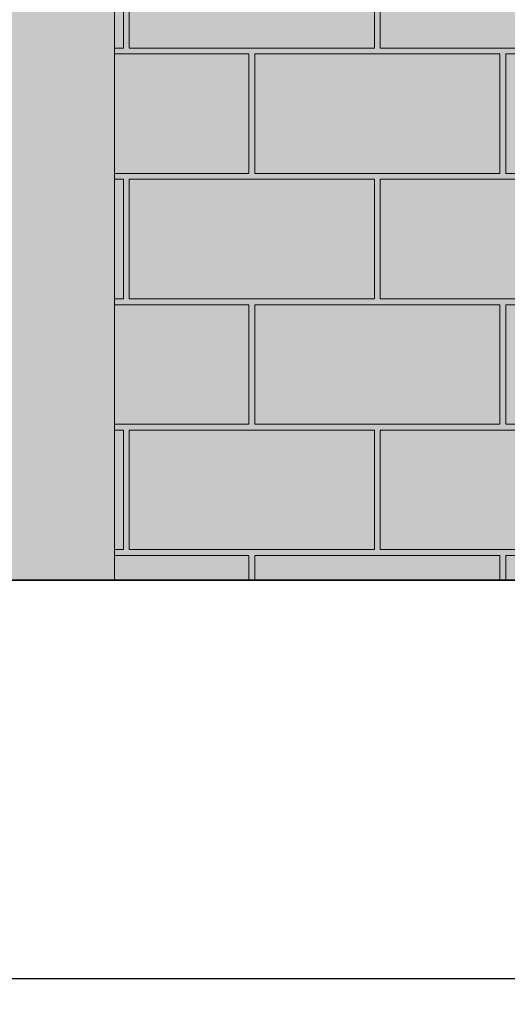
# Model space of a CAD drawing. Units: inches. Extents: x 1704 to 6393, y -157 to 1172.
# Tile 7 of 122: x 1961 to 2035, y -69 to 82. Entities that reach past the tile are written whole.
import ezdxf

# ---------------------------------------------------------------- set-up
doc = ezdxf.new("R2010")
doc.units = ezdxf.units.IN
doc.header["$MEASUREMENT"] = 0
for name, color, linetype, lineweight in [('A-ANNO-DIMS', 7, 'Continuous', 13), ('C-PROP', 7, 'Continuous', 35), ('L-HRDS', 8, 'Continuous', 18), ('L-PVMT-PATT', 8, 'Continuous', 13)]:
    doc.layers.add(name, color=color, linetype=linetype, lineweight=lineweight)
doc.layers.add('L-HRDS-PATT', color=9, linetype='Continuous', lineweight=13, true_color=0xc5c1ba)
doc.layers.add('L-PLNT-PATT', color=253, linetype='Continuous', lineweight=13, true_color=0x9abc8f)
doc.styles.get("Standard").update_dxf_attribs({"font": 'arial.ttf'})
doc.dimstyles.get("Standard").update_dxf_attribs({"dimtxt": 6, "dimasz": 2, "dimexe": 0.18, "dimexo": 0.0625, "dimgap": 0.09, "dimtad": 0, "dimtih": 1, "dimtoh": 1, "dimdec": 1, "dimzin": 0, "dimdsep": 46, "dimlunit": 3, "dimtxsty": 'Standard', "dimblk": 'ARCHTICK', "dimcen": 0.09, "dimadec": 0, "dimazin": 0, "dimtfac": 1, "dimtdec": 1, "dimtofl": 0, "dimtmove": 0, "dimatfit": 3, "dimfxl": 1, "dimtolj": 1, "dimtzin": 0, "dimarcsym": 0})

# ---------------------------------------------------------------- blocks, each defined once
blk = doc.blocks.new('_ArchTick')
at = {"color": 0, "linetype": 'ByBlock', "const_width": 0.15}
blk.add_lwpolyline([(-0.5, -0.5), (0.5, 0.5)], dxfattribs=at)
blk = doc.blocks.new('*D90')
at = {"layer": 'A-ANNO-DIMS', "color": 0, "lineweight": -2, "transparency": 16777216}
for p, q in [((1898.35, -3.85), (1898.35, -64.97)), ((2723.35, -3.85), (2723.35, -64.97)), ((1898.35, -64.79), (2304.1, -64.79)), ((2723.35, -64.79), (2317.59, -64.79))]:
    blk.add_line(p, q, dxfattribs=at)
at = {"layer": 'Defpoints', "color": 0, "lineweight": -3, "transparency": 16777216}
for p in [(1898.35, -3.79), (2723.35, -3.79), (2723.35, -64.79)]:
    blk.add_point(p, dxfattribs=at)
at = {"layer": 'A-ANNO-DIMS', "color": 0, "lineweight": -2, "transparency": 16777216, "xscale": 2, "yscale": 2, "zscale": 2, "rotation": 180}
blk.add_blockref('_ArchTick', (1898.35, -64.79), dxfattribs=at)
at = {"layer": 'A-ANNO-DIMS', "color": 0, "lineweight": -2, "transparency": 16777216, "xscale": 2, "yscale": 2, "zscale": 2}
blk.add_blockref('_ArchTick', (2723.35, -64.79), dxfattribs=at)
at = {"layer": 'A-ANNO-DIMS', "color": 0, "transparency": 16777216, "insert": (2310.85, -64.79), "char_height": 6, "attachment_point": 5}
blk.add_mtext('\\A1;825', dxfattribs=at)

msp = doc.modelspace()

# ---------------------------------------------------------------- hatches: boundary and pattern name
at = {"layer": 'L-HRDS-PATT', "transparency": 33554646}
h = msp.add_hatch(color=256, dxfattribs=at)
h.dxf.hatch_style = 1
h.paths.add_polyline_path([(2273.349, 194.213), (2269.516, 194.213), (2268.215, 194.213), (2230.482, 194.213), (2229.181, 194.213), (2225.349, 194.213), (2049.349, 194.213), (2049.349, 202.213), (1975.349, 202.213), (1975.349, -3.787), (2273.349, -3.787)])
at = {"layer": 'L-PLNT-PATT', "transparency": 33554643}
h = msp.add_hatch(color=256, dxfattribs=at)
h.dxf.hatch_style = 1
h.paths.add_polyline_path([(1975.349, 202.213), (1898.349, 202.213), (1898.349, -3.787), (1975.349, -3.787)])
at = {"layer": 'L-PVMT-PATT', "transparency": 33554643}
h = msp.add_hatch(dxfattribs=at)
h.set_pattern_fill('AR-B816C', color=256, scale=2.4)
h.paths.add_polyline_path([(2273.349, 194.213), (2269.516, 194.213), (2268.215, 194.213), (2230.482, 194.213), (2229.181, 194.213), (2225.349, 194.213), (2049.349, 194.213), (2049.349, 202.213), (1975.349, 202.213), (1975.349, -3.787), (2273.349, -3.787)])

# ---------------------------------------------------------------- linework, layer by layer
at = {"layer": 'C-PROP'}
msp.add_line((2723.349, -3.787), (1898.349, -3.787), dxfattribs=at)
at = {"layer": 'L-HRDS'}
msp.add_line((1975.349, 202.213), (1975.349, -3.787), dxfattribs=at)

# ---------------------------------------------------------------- dimensions: what is measured, and where the dimension line sits
at = {"layer": 'A-ANNO-DIMS'}
dim = msp.add_linear_dim(base=(2723.349, -64.787), p1=(1898.349, -3.787), p2=(2723.349, -3.787), dimstyle='Standard', override={"dimdec": 0, "dimlfac": 1, "dimrnd": 0, "dimzin": 0, "dimdsep": 46, "dimlunit": 2}, dxfattribs=at)
dim.commit()
dim.dimension.update_dxf_attribs({"geometry": '*D90', "text_midpoint": (2310.849, -64.787)})

doc.saveas('drawing.dxf')
